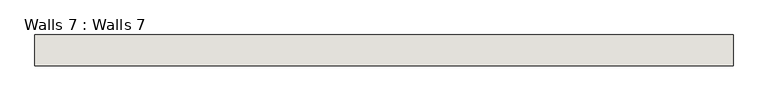
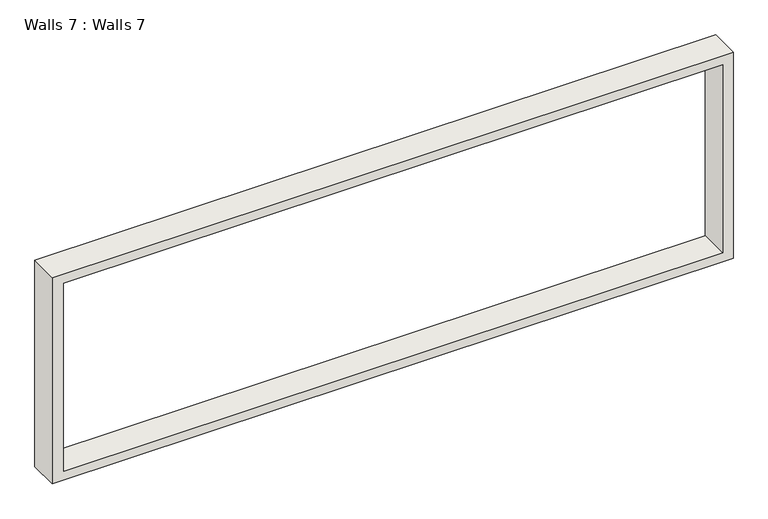
"""IFC4 building model written with IfcOpenShell, lengths in millimetres: wall geometry, Walls 7 : Walls 7."""

from ifc_helpers import new_model, si_unit, frame, origin, place, context, project, spatial, polyline, outline, extrude, source, transform, mapped, element, save


def walls_7_walls_7_225e37e1(model_context):
    return source(origin(), model_context, "Body", "SweptSolid", [
        extrude(outline(polyline([(-152.4, 134.977479), (2133.6, 134.977479), (2133.6, -7004.022521), (-152.4, -7004.022521), (-152.4, 134.977479)]), holes=[polyline([(-54.1554296, 26.8638712), (-54.1554296, -6881.9361288), (2028.6445704, -6881.9361288), (2028.6445704, 26.8638712), (-54.1554296, 26.8638712)])]), frame((0.0, -17642.4049623, 0.0), z_axis=(0.0, 1.0, 0.0), x_axis=(0.0, 0.0, 1.0)), (0.0, 0.0, 1.0), 314.3074626),
    ])


if __name__ == "__main__":
    model = new_model("IFC4")
    model_context = context("Model", 3, world=origin())
    ifc_project = project(units=[si_unit("LENGTHUNIT", "METRE", prefix="MILLI")], contexts=[model_context])
    site = spatial("IfcSite", under=ifc_project)
    building = spatial("IfcBuilding", under=site)
    placement = place(None, origin())
    walls_7_walls_7_shape = walls_7_walls_7_225e37e1(model_context)
    element("IfcWall", 1, ObjectType="Walls 7 : Walls 7", at=placement, inside=building, context=model_context, shape_type="MappedRepresentation", body=[
        mapped(walls_7_walls_7_shape, transform((0.0, 0.0, 0.0), x_axis=(1.0, 0.0, 0.0), y_axis=(0.0, 1.0, 0.0), z_axis=(0.0, 0.0, 1.0))),
    ])
    save(model, "model.ifc")

# Revit data of these elements
# Element 1 (IfcWall, "Walls 7 : Walls 7")
#   Materials on its faces: "Door - Frame", "Default Wall"
# Materials
#   "Door - Frame": colour RGB 118 70 51, transparency 0
#   "Default Wall": colour RGB 128 128 128, transparency 0
